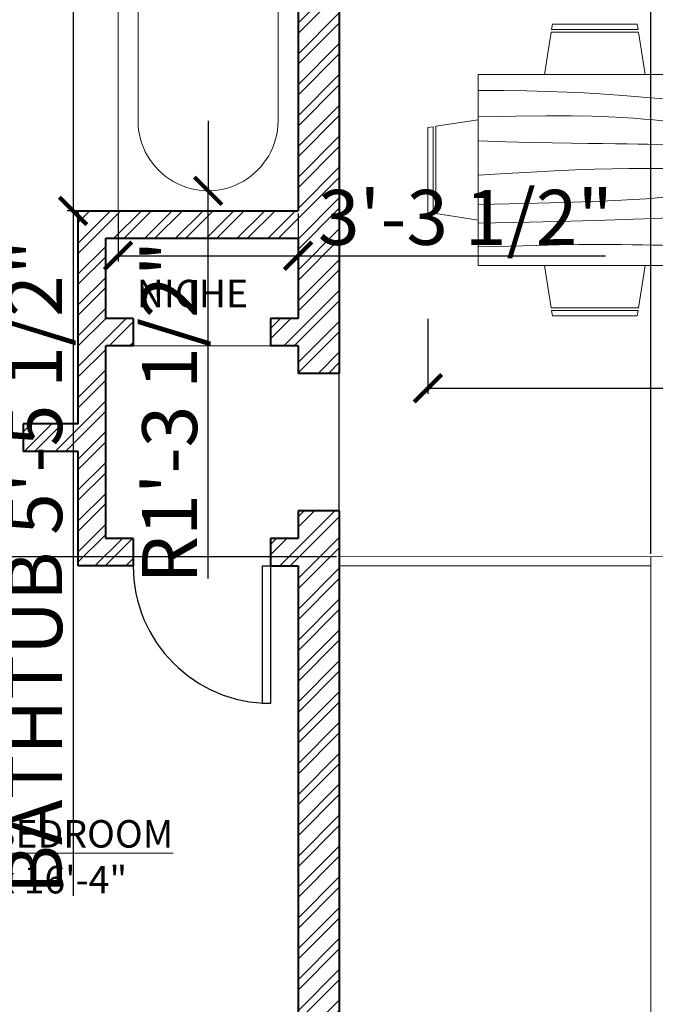
# Model space of a CAD drawing. Units: inches. Extents: x 982 to 1904, y 735 to 1463.
# Tile 3 of 7: x 1301 to 1439, y 945 to 1160. Entities that reach past the tile are written whole.
import ezdxf

# ---------------------------------------------------------------- set-up
doc = ezdxf.new("R2010")
doc.units = ezdxf.units.IN
for name, color, linetype, lineweight in [('A-ANNO-TEXT', 7, 'Continuous', 18), ('A-AREA-IDEN', 7, 'Continuous', 18), ('A-FLOR-CASE', 8, 'Continuous', 20), ('A-FLOR-FIXT', 70, 'Continuous', 20), ('Dimensions', 9, 'Continuous', 18), ('Doors', 130, 'Continuous', 25), ('Furniture', 31, 'Continuous', 18), ('Stairs', 50, 'Continuous', 20), ('Wall Hatch', 23, 'Continuous', 13), ('Walls', 151, 'Continuous', 40)]:
    doc.layers.add(name, color=color, linetype=linetype, lineweight=lineweight)
doc.styles.get("Standard").update_dxf_attribs({"font": 'arial.ttf'})
doc.dimstyles.new('ISO-25', dxfattribs={"dimtxt": 12, "dimasz": 6, "dimexe": 1.25, "dimexo": 0.625, "dimtad": 1, "dimlunit": 3, "dimtxsty": 'Standard', "dimblk": 'ARCHTICK', "dimcen": 2.5, "dimadec": 0, "dimazin": 0, "dimtfac": 1, "dimtmove": 0, "dimatfit": 3, "dimfxl": 1, "dimarcsym": 0})

# ---------------------------------------------------------------- blocks, each defined once
blk = doc.blocks.new('Dining Set - 36 x 72 in.')
for p, q in [((-22.2343, 26.00059), (-23.4847, 17.99762)), ((-22.2304, 26), (-5.7608, 26)), ((-22, 27.5), (-22.1562, 26.50042)), ((-5.8416, 26.5), (-22.1534, 26.5)), ((-22, 27.5), (-6, 27.5)), ((-5.8437, 26.49966), (-6, 27.5)), ((-4.5152, 17.99762), (-5.7655, 25.99926)), ((5.7657, 26.00059), (4.5153, 17.99762)), ((5.7696, 26), (22.2392, 26)), ((6, 27.5), (5.8438, 26.50042)), ((22.1584, 26.5), (5.8466, 26.5)), ((6, 27.5), (22, 27.5)), ((22.1563, 26.49966), (22, 27.5)), ((23.4848, 17.99762), (22.2345, 25.99926)), ((36, 18), (-36, 18)), ((-36, 18), (-36, -18)), ((36, -18), (36, 18)), ((-44.0006, 8.23428), (-35.9976, 9.48474)), ((44.0006, 8.23428), (35.9976, 9.48474)), ((-45.5, 8), (-44.5004, 8.15617)), ((-45.5, 8), (-45.5, -8)), ((-44.5, -8.15843), (-44.5, 8.15338)), ((-44, 8.23041), (-44, -8.23915)), ((44, 8.23041), (44, -8.23915)), ((44.5, -8.15843), (44.5, 8.15338)), ((45.5, 8), (44.5005, 8.15617)), ((45.5, 8), (45.5, -8)), ((-44.4997, -8.15631), (-45.5, -8)), ((-35.9976, -9.48476), (-43.9993, -8.2345)), ((35.9976, -9.48476), (43.9993, -8.2345)), ((44.4997, -8.15631), (45.5, -8)), ((-36, -18), (36, -18)), ((-22.2343, -26.0006), (-23.4847, -17.99762)), ((-4.5152, -17.99762), (-5.7655, -25.99928)), ((5.7657, -26.0006), (4.5153, -17.99762)), ((23.4848, -17.99762), (22.2345, -25.99928)), ((-22.2304, -26), (-5.7608, -26)), ((-22, -27.5), (-22.1562, -26.50044)), ((-5.8416, -26.5), (-22.1534, -26.5)), ((-22, -27.5), (-6, -27.5)), ((-5.8437, -26.49967), (-6, -27.5)), ((5.7696, -26), (22.2392, -26)), ((6, -27.5), (5.8438, -26.50044)), ((22.1584, -26.5), (5.8466, -26.5)), ((6, -27.5), (22, -27.5)), ((22.1563, -26.49967), (22, -27.5))]:
    blk.add_line(p, q)
for points in [[(-36, 15), (-31.1772, 14.97754), (-26.8079, 14.91406), (-22.8538, 14.81543), (-19.276, 14.6875), (-16.0362, 14.53613), (-13.0957, 14.36718), (-10.4159, 14.18652), (-7.9583, 14), (-5.6904, 13.81315), (-3.6035, 13.63021), (-1.6954, 13.45508), (0.0365, 13.29166), (1.5945, 13.14388), (2.9811, 13.01562), (4.1988, 12.9108), (5.25, 12.83333), (6.1393, 12.78613), (6.8802, 12.76823), (7.4883, 12.77767), (7.9792, 12.8125), (8.3685, 12.87077), (8.6719, 12.95052), (8.9049, 13.0498), (9.0833, 13.16666), (9.2205, 13.29899), (9.3216, 13.44401), (9.3895, 13.59879), (9.4271, 13.76041), (9.4373, 13.92594), (9.4232, 14.09245), (9.3875, 14.257), (9.3333, 14.41666), (9.2638, 14.56917), (9.1836, 14.71484), (9.0975, 14.85465), (9.0104, 14.98958), (8.9272, 15.1206), (8.8529, 15.2487), (8.7922, 15.37483), (8.75, 15.5), (8.7305, 15.62467), (8.7344, 15.74739), (8.7617, 15.86621), (8.8125, 15.97916), (8.8867, 16.08431), (8.9844, 16.17968), (9.1055, 16.26334), (9.25, 16.33333), (9.4189, 16.38802), (9.6172, 16.42708), (9.8506, 16.45052), (10.125, 16.45833), (10.4463, 16.45052), (10.8203, 16.42708), (11.2529, 16.38802), (11.75, 16.33333), (12.3184, 16.26318), (12.9694, 16.17838), (13.7151, 16.07991), (14.5677, 15.96875), (15.5395, 15.84586), (16.6426, 15.71224), (17.8893, 15.56884), (19.2917, 15.41666), (20.859, 15.25667), (22.5879, 15.08984), (24.4721, 14.91715), (26.5052, 14.73958), (28.6809, 14.5581), (30.9929, 14.3737), (33.4347, 14.18733), (36, 14)], [(-36, 10), (-28.9766, 10.14274), (-23.1725, 10.20442), (-18.4241, 10.19775), (-14.5677, 10.13541), (-11.4399, 10.03011), (-8.877, 9.89453), (-6.7154, 9.74137), (-4.7917, 9.58333), (-2.9698, 9.43082), (-1.2246, 9.28515), (0.4415, 9.14534), (2.026, 9.01041), (3.5266, 8.87939), (4.9408, 8.7513), (6.266, 8.62516), (7.5, 8.5), (8.6411, 8.37549), (9.6914, 8.2539), (10.6538, 8.13818), (11.5312, 8.03125), (12.3267, 7.93603), (13.043, 7.85547), (13.6831, 7.79248), (14.25, 7.75), (14.7471, 7.7303), (15.1797, 7.73307), (15.5537, 7.75732), (15.875, 7.80208), (16.1494, 7.86637), (16.3828, 7.94922), (16.5811, 8.04964), (16.75, 8.16666), (16.8944, 8.29915), (17.0143, 8.44531), (17.1089, 8.60319), (17.1771, 8.77083), (17.218, 8.94629), (17.2305, 9.1276), (17.2137, 9.31282), (17.1667, 9.5), (17.0895, 9.6875), (16.987, 9.875), (16.8649, 10.0625), (16.7292, 10.25), (16.5856, 10.4375), (16.4401, 10.625), (16.2985, 10.8125), (16.1667, 11), (16.05, 11.18733), (15.9518, 11.3737), (15.8752, 11.5581), (15.8229, 11.73958), (15.798, 11.91715), (15.8034, 12.08984), (15.842, 12.25667), (15.9167, 12.41666), (16.0295, 12.56836), (16.1784, 12.70833), (16.3605, 12.83268), (16.5729, 12.9375), (16.8127, 13.01888), (17.0768, 13.07291), (17.3625, 13.0957), (17.6667, 13.08333), (17.9894, 13.03312), (18.3418, 12.94726), (18.7382, 12.82918), (19.1927, 12.68229), (19.7195, 12.51001), (20.3327, 12.31575), (21.0465, 12.10294), (21.875, 11.875), (22.8357, 11.63354), (23.959, 11.37304), (25.2786, 11.08618), (26.8282, 10.76562), (28.6414, 10.40405), (30.752, 9.99414), (33.1936, 9.52856), (36, 9)], [(-36, 5.5), (-30.7157, 5.3348), (-26.069, 5.20963), (-21.9946, 5.11767), (-18.4271, 5.05208), (-15.3009, 5.00602), (-12.5508, 4.97265), (-10.1112, 4.94515), (-7.9167, 4.91666), (-5.909, 4.88167), (-4.0586, 4.83984), (-2.3429, 4.79215), (-0.7396, 4.73958), (0.7739, 4.6831), (2.22, 4.6237), (3.6213, 4.56233), (5, 4.5), (6.373, 4.43782), (7.7344, 4.3776), (9.0723, 4.32129), (10.375, 4.27083), (11.6309, 4.22819), (12.8281, 4.19531), (13.9551, 4.17415), (15, 4.16666), (15.954, 4.17448), (16.819, 4.19791), (17.6001, 4.23698), (18.3021, 4.29166), (18.9299, 4.36198), (19.4883, 4.44791), (19.9823, 4.54948), (20.4167, 4.66666), (20.7969, 4.79899), (21.1302, 4.94401), (21.4245, 5.09879), (21.6875, 5.26041), (21.9271, 5.42594), (22.1511, 5.59245), (22.3672, 5.757), (22.5834, 5.91666), (22.8065, 6.06868), (23.0404, 6.21093), (23.2879, 6.34147), (23.5521, 6.45833), (23.8358, 6.55957), (24.142, 6.64323), (24.4735, 6.70735), (24.8334, 6.75), (25.2235, 6.76969), (25.642, 6.76692), (26.0858, 6.74267), (26.5521, 6.69791), (27.0379, 6.63362), (27.5404, 6.55078), (28.0565, 6.45036), (28.5834, 6.33333), (29.1242, 6.19987), (29.7071, 6.04687), (30.3661, 5.87044), (31.1354, 5.66666), (32.0493, 5.43164), (33.142, 5.16146), (34.4475, 4.85221), (36, 4.5)], [(-36, -1), (-30.7915, -0.6591), (-26.0195, -0.38216), (-21.6519, -0.16284), (-17.6563, 0.00521), (-14.0005, 0.12833), (-10.6523, 0.21289), (-7.5796, 0.26522), (-4.75, 0.29166), (-2.134, 0.29793), (0.2878, 0.28711), (2.5317, 0.26163), (4.6146, 0.22396), (6.5529, 0.17651), (8.3633, 0.12174), (10.0623, 0.06209), (11.6667, 0), (13.1899, -0.06201), (14.6341, -0.1211), (15.9982, -0.17432), (17.2813, -0.21875), (18.4823, -0.25147), (19.6003, -0.26953), (20.6343, -0.27002), (21.5834, -0.25), (22.4481, -0.20768), (23.2357, -0.14584), (23.9549, -0.06836), (24.6146, 0.02083), (25.2235, 0.11784), (25.7904, 0.21875), (26.3241, 0.31966), (26.8334, 0.41666), (27.3265, 0.50618), (27.8099, 0.58593), (28.2894, 0.65397), (28.7709, 0.70833), (29.2601, 0.74707), (29.763, 0.76823), (30.2855, 0.76985), (30.8334, 0.75), (31.4088, 0.70784), (31.9994, 0.64713), (32.589, 0.57275), (33.1615, 0.48958), (33.7008, 0.4025), (34.1908, 0.3164), (34.6153, 0.23616), (34.9584, 0.16666), (35.2099, 0.11165), (35.3848, 0.07031), (35.504, 0.04069), (35.5886, 0.02083), (35.6594, 0.00879), (35.7377, 0.0026), (35.8442, 0.00032), (36, 0)], [(-36, -6.5), (-27.1843, -6.31267), (-20.084, -6.1263), (-14.469, -5.9419), (-10.1094, -5.76042), (-6.7752, -5.58285), (-4.2363, -5.41016), (-2.2629, -5.24333), (-0.625, -5.08334), (0.8708, -4.93099), (2.2715, -4.78646), (3.5872, -4.64974), (4.8281, -4.52084), (6.0046, -4.39974), (7.127, -4.28646), (8.2053, -4.18099), (9.25, -4.08334), (10.2705, -3.99382), (11.2734, -3.91407), (12.2647, -3.84603), (13.25, -3.79167), (14.2354, -3.75293), (15.2266, -3.73177), (16.2295, -3.73015), (17.25, -3.75), (18.2912, -3.79248), (19.3451, -3.85547), (20.4009, -3.93604), (21.4479, -4.03125), (22.4754, -4.13819), (23.4727, -4.25391), (24.4289, -4.37549), (25.3334, -4.5), (26.1785, -4.62492), (26.9694, -4.74935), (27.7145, -4.87281), (28.4219, -4.99479), (29.1, -5.11483), (29.7572, -5.23242), (30.4016, -5.34709), (31.0417, -5.45834), (31.6837, -5.56437), (32.3262, -5.65821), (32.9658, -5.73153), (33.599, -5.77604), (34.2224, -5.78345), (34.8327, -5.74545), (35.4264, -5.65373), (36, -5.5)], [(-36, -10), (-26.4022, -9.81299), (-18.4675, -9.62891), (-11.9839, -9.45069), (-6.7396, -9.28125), (-2.5226, -9.12354), (0.8789, -8.98047), (3.6769, -8.85498), (6.0833, -8.75), (8.2767, -8.66765), (10.3021, -8.60677), (12.1712, -8.56543), (13.8958, -8.54167), (15.4876, -8.53353), (16.9583, -8.53907), (18.3197, -8.55632), (19.5834, -8.58334), (20.7616, -8.61841), (21.8685, -8.66081), (22.9188, -8.71004), (23.9271, -8.76563), (24.9081, -8.82707), (25.8763, -8.89388), (26.8465, -8.96558), (27.8334, -9.04167), (28.8474, -9.12118), (29.8828, -9.20117), (30.93, -9.27824), (31.9792, -9.34896), (33.0205, -9.40991), (34.0443, -9.45768), (35.0407, -9.48885), (36, -9.5)], [(-36, -14.5), (-30.0881, -14.33513), (-25.0332, -14.21224), (-20.7312, -14.12647), (-17.0781, -14.07292), (-13.97, -14.04671), (-11.3027, -14.04297), (-8.9724, -14.05681), (-6.875, -14.08334), (-4.9224, -14.11833), (-3.0905, -14.16016), (-1.3709, -14.20785), (0.2448, -14.26042), (1.7647, -14.3169), (3.1973, -14.3763), (4.5507, -14.43767), (5.8333, -14.5), (7.0554, -14.5621), (8.235, -14.62175), (9.3922, -14.67652), (10.5469, -14.72396), (11.7192, -14.76164), (12.929, -14.78711), (14.1965, -14.79794), (15.5417, -14.79167), (16.9933, -14.76424), (18.6152, -14.70508), (20.4804, -14.60197), (22.6615, -14.44271), (25.2312, -14.21509), (28.2624, -13.9069), (31.8277, -13.50594), (36, -13)]]:
    blk.add_lwpolyline(points)
blk = doc.blocks.new('Bath Tub - 26 x 60 in.')
for p, q in [((9, -17), (9, -19)), ((8, -18), (10, -18))]:
    blk.add_line(p, q)
blk.add_lwpolyline([(0, -36), (0, 0), (60, 0), (60, -36)], close=True)
for points in [[(6, -4), (42, -4)], [(4, -30), (4, -6)], [(42, -32), (6, -32)]]:
    blk.add_lwpolyline(points)
for radius in [1.5, 1]:
    blk.add_circle((9, -18), radius)
for centre, radius, start, end in [((5.75, -5.75), 1.77, 81.8699, 188.1301), ((42, -18), 14, 270, 90), ((5.75, -30.25), 1.77, 171.8699, 278.1301)]:
    blk.add_arc(centre, radius, start, end)
blk = doc.blocks.new('*U21')
for p, q in [((-750, 0), (-750, 100)), ((0, 0), (0, 100))]:
    blk.add_line(p, q)
blk.add_lwpolyline([(0, 0), (0, -750), (-43.75, -750), (-43.75, 0)], close=True)
blk.add_arc((0, 0), 750, 180, 270)
blk = doc.blocks.new('_ArchTick')
at = {"color": 0, "linetype": 'ByBlock', "const_width": 0.15}
blk.add_lwpolyline([(-0.5, -0.5), (0.5, 0.5)], dxfattribs=at)
blk = doc.blocks.new('*D40')
at = {"layer": 'Defpoints', "color": 0, "transparency": 16777216}
for p in [(1389.84, 1095.57), (1495.17, 1095.57), (1495.17, 1079.77)]:
    blk.add_point(p, dxfattribs=at)
at = {"layer": 'Dimensions', "color": 0, "lineweight": -2, "transparency": 16777216}
for p, q in [((1389.84, 1094.94), (1389.84, 1078.52)), ((1495.17, 1094.94), (1495.17, 1078.52)), ((1389.84, 1079.77), (1495.17, 1079.77)), ((1495.17, 1079.77), (1662.27, 1079.77))]:
    blk.add_line(p, q, dxfattribs=at)
at = {"layer": 'Dimensions', "color": 0, "lineweight": -2, "transparency": 16777216, "xscale": 6, "yscale": 6, "zscale": 6, "rotation": 180}
blk.add_blockref('_ArchTick', (1389.84, 1079.77), dxfattribs=at)
at = {"layer": 'Dimensions', "color": 0, "lineweight": -2, "transparency": 16777216, "xscale": 6, "yscale": 6, "zscale": 6}
blk.add_blockref('_ArchTick', (1495.17, 1079.77), dxfattribs=at)
at = {"layer": 'Dimensions', "color": 0, "transparency": 16777216, "insert": (1581.72, 1086.6), "char_height": 12, "attachment_point": 5}
blk.add_mtext('DINING SET 8\'-9 1/2"', dxfattribs=at)
blk = doc.blocks.new('*D52')
at = {"layer": 'Defpoints', "color": 0, "transparency": 16777216}
for p in [(1322.2, 1183.99), (1312.37, 1118.49), (1322.2, 1118.49)]:
    blk.add_point(p, dxfattribs=at)
at = {"layer": 'Dimensions', "color": 0, "lineweight": -2, "transparency": 16777216}
for p, q in [((1321.57, 1183.99), (1311.12, 1183.99)), ((1312.37, 1183.99), (1312.37, 1118.49)), ((1321.57, 1118.49), (1311.12, 1118.49)), ((1312.37, 1118.49), (1312.37, 969.02))]:
    blk.add_line(p, q, dxfattribs=at)
at = {"layer": 'Dimensions', "color": 0, "lineweight": -2, "transparency": 16777216, "xscale": 6, "yscale": 6, "zscale": 6}
for p, rotation in [((1312.37, 1183.99), 90), ((1312.37, 1118.49), 270)]:
    blk.add_blockref('_ArchTick', p, dxfattribs=dict(at, rotation=rotation))
at = {"layer": 'Dimensions', "color": 0, "transparency": 16777216, "insert": (1305.54, 1040.75), "char_height": 12, "attachment_point": 5, "rotation": 90}
blk.add_mtext('BATHTUB 5\'-5 1/2"', dxfattribs=at)
blk = doc.blocks.new('*D53')
at = {"layer": 'Defpoints', "color": 0, "transparency": 16777216}
for p in [(1322.2, 1118.49), (1361.5, 1118.49), (1361.5, 1108.67)]:
    blk.add_point(p, dxfattribs=at)
at = {"layer": 'Dimensions', "color": 0, "lineweight": -2, "transparency": 16777216}
for p, q in [((1322.2, 1117.87), (1322.2, 1107.42)), ((1361.5, 1117.87), (1361.5, 1107.42)), ((1322.2, 1108.67), (1361.5, 1108.67)), ((1361.5, 1108.67), (1428.6, 1108.67))]:
    blk.add_line(p, q, dxfattribs=at)
at = {"layer": 'Dimensions', "color": 0, "lineweight": -2, "transparency": 16777216, "xscale": 6, "yscale": 6, "zscale": 6, "rotation": 180}
blk.add_blockref('_ArchTick', (1322.2, 1108.67), dxfattribs=at)
at = {"layer": 'Dimensions', "color": 0, "lineweight": -2, "transparency": 16777216, "xscale": 6, "yscale": 6, "zscale": 6}
blk.add_blockref('_ArchTick', (1361.5, 1108.67), dxfattribs=at)
at = {"layer": 'Dimensions', "color": 0, "transparency": 16777216, "insert": (1398.05, 1115.5), "char_height": 12, "attachment_point": 5}
blk.add_mtext('3\'-3 1/2"', dxfattribs=at)
blk = doc.blocks.new('*D64')
at = {"layer": 'Defpoints', "color": 0, "transparency": 16777216}
for p in [(1482.5, 1427.79), (1370.5, 841.99), (1482.5, 841.99)]:
    blk.add_point(p, dxfattribs=at)
at = {"layer": 'Dimensions', "color": 0, "lineweight": -2, "transparency": 16777216}
for p, q in [((1370.5, 842.62), (1370.5, 1429.04)), ((1482.5, 842.62), (1482.5, 1429.04)), ((1370.5, 1427.79), (1482.5, 1427.79))]:
    blk.add_line(p, q, dxfattribs=at)
at = {"layer": 'Dimensions', "color": 0, "lineweight": -2, "transparency": 16777216, "xscale": 6, "yscale": 6, "zscale": 6, "rotation": 180}
blk.add_blockref('_ArchTick', (1370.5, 1427.79), dxfattribs=at)
at = {"layer": 'Dimensions', "color": 0, "lineweight": -2, "transparency": 16777216, "xscale": 6, "yscale": 6, "zscale": 6}
blk.add_blockref('_ArchTick', (1482.5, 1427.79), dxfattribs=at)
at = {"layer": 'Dimensions', "color": 0, "transparency": 16777216, "insert": (1426.5, 1434.54), "char_height": 12, "attachment_point": 5}
blk.add_mtext('9\'-4"', dxfattribs=at)
blk = doc.blocks.new('*D65')
at = {"layer": 'Defpoints', "color": 0, "transparency": 16777216}
for p in [(1123.7, 1042.99), (1370.5, 1042.99), (1370.5, 841.99)]:
    blk.add_point(p, dxfattribs=at)
at = {"layer": 'Dimensions', "color": 0, "lineweight": -2, "transparency": 16777216}
for p, q in [((1369.87, 1042.99), (1122.45, 1042.99)), ((1123.7, 841.99), (1123.7, 1042.99)), ((1369.87, 841.99), (1122.45, 841.99))]:
    blk.add_line(p, q, dxfattribs=at)
at = {"layer": 'Dimensions', "color": 0, "lineweight": -2, "transparency": 16777216, "xscale": 6, "yscale": 6, "zscale": 6}
for p, rotation in [((1123.7, 1042.99), 90), ((1123.7, 841.99), 270)]:
    blk.add_blockref('_ArchTick', p, dxfattribs=dict(at, rotation=rotation))
at = {"layer": 'Dimensions', "color": 0, "transparency": 16777216, "insert": (1116.94, 942.49), "char_height": 12, "attachment_point": 5, "rotation": 90}
blk.add_mtext('16\'-9"', dxfattribs=at)
blk = doc.blocks.new('*D66')
at = {"layer": 'Defpoints', "color": 0, "transparency": 16777216}
for p in [(1482.5, 1427.79), (1438.5, 1043.01), (1482.5, 1043.03)]:
    blk.add_point(p, dxfattribs=at)
at = {"layer": 'Dimensions', "color": 0, "lineweight": -2, "transparency": 16777216}
for p, q in [((1438.5, 1043.64), (1438.5, 1429.04)), ((1482.5, 1043.65), (1482.5, 1429.04)), ((1438.5, 1427.79), (1482.5, 1427.79))]:
    blk.add_line(p, q, dxfattribs=at)
at = {"layer": 'Dimensions', "color": 0, "lineweight": -2, "transparency": 16777216, "xscale": 6, "yscale": 6, "zscale": 6, "rotation": 180}
blk.add_blockref('_ArchTick', (1438.5, 1427.79), dxfattribs=at)
at = {"layer": 'Dimensions', "color": 0, "lineweight": -2, "transparency": 16777216, "xscale": 6, "yscale": 6, "zscale": 6}
blk.add_blockref('_ArchTick', (1482.5, 1427.79), dxfattribs=at)
at = {"layer": 'Dimensions', "color": 0, "transparency": 16777216, "insert": (1460.5, 1434.55), "char_height": 12, "attachment_point": 5}
blk.add_mtext('3\'-8"', dxfattribs=at)
blk = doc.blocks.new('*D75')
at = {"layer": 'Defpoints', "color": 0, "transparency": 16777216}
for p in [(1296.83, 918.98), (1348.87, 866.93)]:
    blk.add_point(p, dxfattribs=at)
at = {"layer": 'Dimensions', "color": 0, "lineweight": -2, "transparency": 16777216}
for p in [(1218.63, 997.17), (1348.87, 866.93)]:
    blk.add_line(p, (1296.83, 918.98), dxfattribs=at)
at = {"layer": 'Dimensions', "color": 0, "lineweight": -2, "transparency": 16777216, "xscale": 6, "yscale": 6, "zscale": 6, "rotation": 314.9994011111431}
blk.add_blockref('_ArchTick', (1296.83, 918.98), dxfattribs=at)
at = {"layer": 'Dimensions', "color": 0, "transparency": 16777216, "insert": (1258.32, 967.15), "char_height": 12, "attachment_point": 5, "rotation": 314.9994}
blk.add_mtext('2X R6\'-1 1/2"', dxfattribs=at)
blk = doc.blocks.new('*D78')
at = {"layer": 'Defpoints', "color": 0, "transparency": 16777216}
for p in [(1341.85, 1138.14), (1341.85, 1122.86)]:
    blk.add_point(p, dxfattribs=at)
at = {"layer": 'Dimensions', "color": 0, "lineweight": -2, "transparency": 16777216}
for p in [(1341.85, 1138.14), (1341.84, 1038.26)]:
    blk.add_line(p, (1341.85, 1122.86), dxfattribs=at)
at = {"layer": 'Dimensions', "color": 0, "lineweight": -2, "transparency": 16777216, "xscale": 6, "yscale": 6, "zscale": 6, "rotation": 89.99842171065775}
blk.add_blockref('_ArchTick', (1341.85, 1122.86), dxfattribs=at)
at = {"layer": 'Dimensions', "color": 0, "transparency": 16777216, "insert": (1335.01, 1074.56), "char_height": 12, "attachment_point": 5, "rotation": 89.9984}
blk.add_mtext('R1\'-3 1/2"', dxfattribs=at)

msp = doc.modelspace()

# ---------------------------------------------------------------- hatches: boundary and pattern name
at = {"layer": 'Wall Hatch'}
h = msp.add_hatch(dxfattribs=at)
h.set_pattern_fill('ANSI32', color=256, scale=0.5)
h.paths.add_polyline_path([(1165.496, 1065.991), (1271.496, 1065.991), (1271.496, 1071.991), (1218.496, 1071.991), (1218.496, 1238.491), (1262.496, 1238.491), (1262.496, 1244.491), (1218.496, 1244.491), (1218.496, 1330.491), (1298.496, 1330.491), (1298.496, 1244.491), (1292.496, 1244.491), (1292.496, 1238.491), (1298.496, 1238.491), (1298.496, 1221.991), (1304.496, 1221.991), (1304.496, 1224.991), (1374.496, 1224.991), (1374.496, 1230.991), (1304.496, 1230.991), (1304.496, 1251.991), (1310.496, 1251.991), (1310.496, 1257.991), (1304.496, 1257.991), (1304.496, 1385.991), (1328.496, 1385.991), (1328.496, 1394.991), (1295.496, 1394.991), (1295.496, 1339.491), (1209.496, 1339.491), (1209.496, 1071.991), (1156.496, 1071.991), (1156.496, 893.991), (1171.496, 893.991), (1171.496, 902.991), (1165.496, 902.991)])
h.paths.add_polyline_path([(1273.996, 877.991), (1267.996, 877.991), (1267.996, 902.991), (1252.996, 902.991), (1252.996, 893.991), (1258.996, 893.991), (1258.996, 868.991), (1273.996, 868.991)])
h.paths.add_polyline_path([(1370.496, 1052.991), (1361.496, 1052.991), (1361.496, 1046.991), (1355.496, 1046.991), (1355.496, 1040.991), (1361.496, 1040.991), (1361.496, 877.991), (1355.496, 877.991), (1355.496, 868.991), (1361.496, 868.991), (1361.496, 832.991), (1376.313, 832.991), (1491.496, 832.991), (1491.496, 985.991), (1515.496, 985.991), (1515.496, 994.991), (1482.496, 994.991), (1482.496, 841.991), (1370.496, 841.991)])
h.paths.add_polyline_path([(1319.496, 1088.991), (1325.496, 1088.991), (1325.496, 1094.991), (1319.496, 1094.991), (1319.496, 1112.491), (1361.496, 1112.491), (1361.496, 1094.991), (1355.496, 1094.991), (1355.496, 1088.991), (1361.496, 1088.991), (1361.496, 1082.991), (1370.496, 1082.991), (1370.496, 1180.991), (1503.496, 1180.991), (1503.496, 1231.991), (1497.496, 1231.991), (1497.496, 1215.991), (1491.496, 1215.991), (1491.496, 1209.991), (1497.496, 1209.991), (1497.496, 1189.991), (1448.496, 1189.991), (1448.496, 1209.991), (1454.496, 1209.991), (1454.496, 1215.991), (1448.496, 1215.991), (1448.496, 1221.991), (1442.496, 1221.991), (1442.496, 1189.991), (1380.496, 1189.991), (1380.496, 1251.991), (1442.496, 1251.991), (1442.496, 1245.991), (1448.496, 1245.991), (1448.496, 1263.991), (1442.496, 1263.991), (1442.496, 1257.991), (1368.496, 1257.991), (1368.496, 1251.991), (1374.496, 1251.991), (1374.496, 1189.991), (1304.496, 1189.991), (1304.496, 1192.991), (1295.496, 1192.991), (1295.496, 1183.991), (1361.496, 1183.991), (1361.496, 1118.491), (1313.496, 1118.491), (1313.496, 1071.991), (1301.496, 1071.991), (1301.496, 1065.991), (1313.496, 1065.991), (1313.496, 1040.991), (1325.496, 1040.991), (1325.496, 1046.991), (1319.496, 1046.991)])
h.paths.add_polyline_path([(1565.496, 1394.991), (1418.496, 1394.991), (1418.496, 1385.991), (1442.496, 1385.991), (1442.496, 1293.991), (1448.496, 1293.991), (1448.496, 1299.991), (1454.496, 1299.991), (1454.496, 1305.991), (1448.496, 1305.991), (1448.496, 1385.991), (1556.496, 1385.991), (1556.496, 1307.991), (1497.496, 1307.991), (1497.496, 1305.991), (1491.496, 1305.991), (1491.496, 1299.991), (1497.496, 1299.991), (1497.496, 1268.991), (1503.496, 1268.991), (1503.496, 1298.991), (1656.496, 1298.991), (1656.496, 1307.991), (1565.496, 1307.991)])
h.paths.add_polyline_path([(1731.496, 1307.991), (1698.496, 1307.991), (1698.496, 1298.991), (1722.496, 1298.991), (1722.496, 1033.991), (1731.496, 1033.991)])
h.paths.add_polyline_path([(1731.496, 997.991), (1722.496, 997.991), (1722.496, 994.991), (1689.496, 994.991), (1689.496, 985.991), (1731.496, 985.991)])

# ---------------------------------------------------------------- linework, layer by layer
at = {"layer": 'A-FLOR-CASE'}
msp.add_line((1325.496, 1088.991), (1355.496, 1088.991), dxfattribs=at)
at = {"layer": 'Stairs'}
for p, q in [((1370.496, 1042.991), (1484.496, 1043.026)), ((1438.496, 1043.012), (1438.496, 886.991)), ((1370.496, 1040.991), (1438.496, 1040.991))]:
    msp.add_line(p, q, dxfattribs=at)
at = {"layer": 'Walls'}
for p, q in [((1361.496, 1183.991), (1361.496, 1118.491)), ((1370.496, 1180.991), (1370.496, 1082.991)), ((1313.496, 1118.491), (1361.496, 1118.491)), ((1313.496, 1071.991), (1313.496, 1118.491)), ((1319.496, 1112.491), (1361.496, 1112.491)), ((1319.496, 1094.991), (1319.496, 1112.491)), ((1361.496, 1112.491), (1361.496, 1094.991)), ((1325.496, 1094.991), (1319.496, 1094.991)), ((1325.496, 1094.991), (1325.496, 1088.991)), ((1361.496, 1094.991), (1355.496, 1094.991)), ((1355.496, 1094.991), (1355.496, 1088.991)), ((1319.496, 1046.991), (1319.496, 1088.991)), ((1325.496, 1088.991), (1319.496, 1088.991)), ((1361.496, 1088.991), (1355.496, 1088.991)), ((1361.496, 1088.991), (1361.496, 1082.991)), ((1370.496, 1082.991), (1361.496, 1082.991)), ((1313.496, 1071.991), (1301.496, 1071.991)), ((1301.496, 1071.991), (1301.496, 1065.991)), ((1313.496, 1065.991), (1301.496, 1065.991)), ((1313.496, 1040.991), (1313.496, 1065.991)), ((1370.496, 1052.991), (1361.496, 1052.991)), ((1361.496, 1052.991), (1361.496, 1046.991)), ((1370.496, 1052.991), (1370.496, 841.991)), ((1325.496, 1046.991), (1319.496, 1046.991)), ((1325.496, 1046.991), (1325.496, 1040.991)), ((1361.496, 1046.991), (1355.496, 1046.991)), ((1355.496, 1046.991), (1355.496, 1040.991)), ((1361.496, 1046.991), (1355.496, 1046.991)), ((1325.496, 1040.991), (1313.496, 1040.991)), ((1355.496, 1040.991), (1361.496, 1040.991)), ((1361.496, 1040.991), (1361.496, 877.991))]:
    msp.add_line(p, q, dxfattribs=at)

# ---------------------------------------------------------------- block references
at = {"layer": 'A-FLOR-FIXT', "xscale": 1.091666666666662, "yscale": 1.091666666666662, "zscale": 1.091666666666662, "rotation": 270}
msp.add_blockref('Bath Tub - 26 x 60 in.', (1361.496, 1183.991), dxfattribs=at)
at = {"layer": 'Doors', "xscale": 0.0399999999999999, "yscale": 0.0399999999999999, "zscale": 0.0399999999999999}
msp.add_blockref('*U21', (1355.496, 1040.991), dxfattribs=at)
at = {"layer": 'Furniture', "xscale": 1.157465785560688, "yscale": 1.157465785560688, "zscale": 1.157465785560688}
msp.add_blockref('Dining Set - 36 x 72 in.', (1442.505, 1127.4), dxfattribs=at)

# ---------------------------------------------------------------- texts
at = {"layer": 'A-ANNO-TEXT', "insert": (1326.273, 1103.43), "char_height": 6, "attachment_point": 1}
msp.add_mtext_dynamic_manual_height_columns('{\\fTimes New Roman|b0|i0|c0|p18;NICHE}', width=30.01819, gutter_width=12.5, heights=[0], dxfattribs=at)
at = {"layer": 'A-AREA-IDEN', "insert": (1255.855, 985.512), "char_height": 6, "attachment_point": 1}
msp.add_mtext_dynamic_manual_height_columns('\\pxqc;{\\fTimes New Roman|b0|i0|c0|p18;\\LMASTER BEDROOM\\P\\l13\'-7" x 16\'-4"}', width=83.67881, gutter_width=12.5, heights=[0], dxfattribs=at)

# ---------------------------------------------------------------- dimensions: what is measured, and where the dimension line sits
at = {"layer": 'Dimensions'}
for base, p1, p2, picture, middle in [((1482.496, 1427.791), (1370.496, 841.991), (1482.496, 841.991), '*D64', (1426.496, 1434.543)), ((1482.496, 1427.791), (1438.496, 1043.012), (1482.496, 1043.025), '*D66', (1460.496, 1434.547)), ((1361.496, 1108.666), (1322.196, 1118.491), (1361.496, 1118.491), '*D53', (1398.048, 1115.5))]:
    dim = msp.add_linear_dim(base=base, p1=p1, p2=p2, dimstyle='ISO-25', override={"dimdec": 1, "dimlfac": 1, "dimrnd": 0, "dimzin": 1, "dimdsep": 46, "dimlunit": 4, "dimfrac": 2}, dxfattribs=at)
    dim.commit()
    dim.dimension.update_dxf_attribs({"geometry": picture, "text_midpoint": middle})
dim = msp.add_linear_dim(base=(1312.371, 1118.491), p1=(1322.196, 1183.991), p2=(1322.196, 1118.491), angle=270, text='BATHTUB <>', dimstyle='ISO-25', override={"dimdec": 1, "dimlfac": 1, "dimrnd": 0, "dimzin": 1, "dimdsep": 46, "dimlunit": 4, "dimfrac": 2}, dxfattribs=at)
dim.commit()
dim.dimension.update_dxf_attribs({"geometry": '*D52', "text_midpoint": (1305.542, 1040.754)})
dim = msp.add_radius_dim(center=(1341.846, 1138.141), mpoint=(1341.846, 1122.858), dimstyle='ISO-25', override={"dimdec": 1, "dimlfac": 1, "dimrnd": 0, "dimzin": 1, "dimdsep": 46, "dimlunit": 4, "dimfrac": 2}, dxfattribs=at)
dim.commit()
dim.dimension.update_dxf_attribs({"geometry": '*D78', "text_midpoint": (1335.011, 1074.56)})
dim = msp.add_linear_dim(base=(1495.169, 1079.77), p1=(1389.84, 1095.569), p2=(1495.169, 1095.569), text='DINING SET <>', dimstyle='ISO-25', override={"dimdec": 1, "dimlfac": 1, "dimrnd": 0, "dimzin": 1, "dimdsep": 46, "dimlunit": 4, "dimfrac": 2}, dxfattribs=at)
dim.commit()
dim.dimension.update_dxf_attribs({"geometry": '*D40', "text_midpoint": (1581.722, 1086.6)})
dim = msp.add_linear_dim(base=(1123.696, 1042.991), p1=(1370.496, 841.991), p2=(1370.496, 1042.991), angle=90, dimstyle='ISO-25', override={"dimdec": 1, "dimlfac": 1, "dimrnd": 0, "dimzin": 1, "dimdsep": 46, "dimlunit": 4, "dimfrac": 2}, dxfattribs=at)
dim.commit()
dim.dimension.update_dxf_attribs({"geometry": '*D65', "text_midpoint": (1116.945, 942.491)})
dim = msp.add_radius_dim(center=(1348.87, 866.934), mpoint=(1296.826, 918.979), text='2X <>', dimstyle='ISO-25', override={"dimdec": 1, "dimlfac": 1, "dimrnd": 0, "dimzin": 1, "dimdsep": 46, "dimlunit": 4, "dimfrac": 2}, dxfattribs=at)
dim.commit()
dim.dimension.update_dxf_attribs({"geometry": '*D75', "text_midpoint": (1258.316, 967.149)})

doc.saveas('drawing.dxf')
